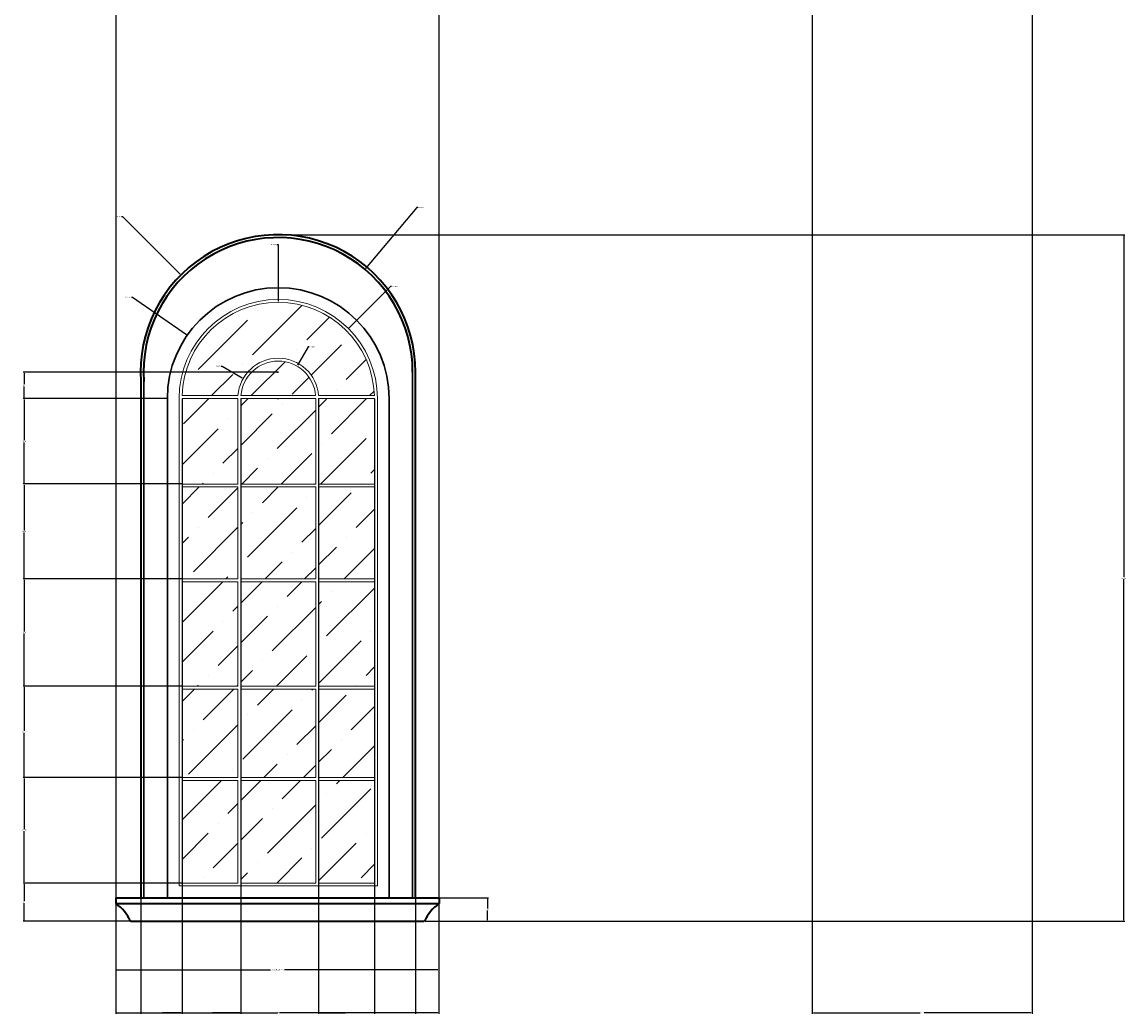
# Model space of a CAD drawing. Units: inches. Extents: x 386 to 708, y 151 to 489.
# Tile 2 of 4: x 520 to 708, y 151 to 320. Entities that reach past the tile are written whole.
import ezdxf

# ---------------------------------------------------------------- set-up
doc = ezdxf.new("R2010")
doc.units = ezdxf.units.IN
doc.header["$MEASUREMENT"] = 0
for name, color, linetype, lineweight in [('A-ANNO-DIMS', 2, 'Continuous', 18), ('A-GLAZ-FRAM', 4, 'Continuous', 30), ('A-GLAZ-PATT', 252, 'Continuous', 13), ('A-GLAZ-SASH', 4, 'Continuous', 18), ('A-GLAZ-SILL', 7, 'Continuous', 35), ('A-GLAZ-TRIM', 7, 'Continuous', 35)]:
    doc.layers.add(name, color=color, linetype=linetype, lineweight=lineweight)
doc.styles.get("Standard").update_dxf_attribs({"font": 'arial.ttf'})
doc.dimstyles.get("Standard").update_dxf_attribs({"dimtxt": 0.18, "dimasz": 0.18, "dimexe": 0.18, "dimexo": 0.0625, "dimgap": 0.09, "dimtad": 0, "dimtih": 1, "dimtoh": 1, "dimdec": 4, "dimzin": 0, "dimdsep": 46, "dimtxsty": 'Standard', "dimcen": 0.09, "dimadec": 0, "dimazin": 0, "dimtfac": 1, "dimtdec": 4, "dimtofl": 0, "dimtmove": 0, "dimatfit": 3, "dimfxl": 1, "dimtolj": 1, "dimtzin": 0, "dimarcsym": 0})

# ---------------------------------------------------------------- blocks, each defined once
blk = doc.blocks.new('WIN-SILL-DOUBLE')
for p, q in [((0, 4), (54.98, 4)), ((0, 4), (0, 3)), ((54.98, 4), (54.98, 3)), ((0, 3), (54.98, 3)), ((2.49, 0), (52.48, 0))]:
    blk.add_line(p, q)
blk.add_lwpolyline([(4.75, 0), (50.49, 0)])
for centre, start, end in [((-4.74, -3.48), 25.6893, 53.8074), ((59.72, -3.48), 126.1926, 154.3107)]:
    blk.add_arc(centre, 8.03, start, end)
blk = doc.blocks.new('*D18')
at = {"layer": 'A-ANNO-DIMS', "color": 0, "lineweight": -2, "transparency": 16777216}
for p, q in [((535.99, 167.19), (535.99, 158.82)), ((590.97, 167.19), (590.97, 158.82)), ((536.17, 159), (562.29, 159)), ((590.79, 159), (564.67, 159))]:
    blk.add_line(p, q, dxfattribs=at)
at = {"layer": 'A-ANNO-DIMS', "color": 0, "transparency": 16777216}
for points in [[(536.17, 159.03), (536.17, 158.97), (535.99, 159)], [(590.79, 159.03), (590.79, 158.97), (590.97, 159)]]:
    blk.add_solid(points, dxfattribs=at)
at = {"layer": 'Defpoints', "color": 0, "transparency": 16777216}
for p in [(535.99, 167.25), (590.97, 167.25), (590.97, 159)]:
    blk.add_point(p, dxfattribs=at)
at = {"layer": 'A-ANNO-DIMS', "color": 0, "transparency": 16777216, "insert": (563.48, 159), "char_height": 0.18, "attachment_point": 5}
blk.add_mtext('\\A1;WIDE SILL 55 TYP.', dxfattribs=at)
blk = doc.blocks.new('*D19')
at = {"layer": 'A-ANNO-DIMS', "color": 0, "lineweight": -2, "transparency": 16777216}
for p, q in [((591.03, 171.25), (599.4, 171.25)), ((599.22, 171.07), (599.22, 169.43)), ((591.03, 167.25), (599.4, 167.25)), ((599.22, 167.43), (599.22, 169.07))]:
    blk.add_line(p, q, dxfattribs=at)
at = {"layer": 'A-ANNO-DIMS', "color": 0, "transparency": 16777216}
for points in [[(599.19, 171.07), (599.25, 171.07), (599.22, 171.25)], [(599.19, 167.43), (599.25, 167.43), (599.22, 167.25)]]:
    blk.add_solid(points, dxfattribs=at)
at = {"layer": 'Defpoints', "color": 0, "transparency": 16777216}
for p in [(590.97, 171.25), (599.22, 171.25), (590.97, 167.25)]:
    blk.add_point(p, dxfattribs=at)
at = {"layer": 'A-ANNO-DIMS', "color": 0, "transparency": 16777216, "insert": (599.22, 169.25), "char_height": 0.18, "attachment_point": 5}
blk.add_mtext('\\A1;4 TYP.', dxfattribs=at)
blk = doc.blocks.new('*D47')
at = {"layer": 'A-ANNO-DIMS', "color": 0, "lineweight": -2, "transparency": 16777216}
for p, q in [((535.99, 370.64), (535.99, 151.47)), ((590.97, 370.64), (590.97, 151.47)), ((536.17, 151.65), (563.09, 151.65)), ((590.79, 151.65), (563.87, 151.65))]:
    blk.add_line(p, q, dxfattribs=at)
at = {"layer": 'A-ANNO-DIMS', "color": 0, "transparency": 16777216}
for points in [[(536.17, 151.68), (536.17, 151.62), (535.99, 151.65)], [(590.79, 151.68), (590.79, 151.62), (590.97, 151.65)]]:
    blk.add_solid(points, dxfattribs=at)
at = {"layer": 'Defpoints', "color": 0, "transparency": 16777216}
for p in [(535.99, 370.7), (590.97, 370.7), (590.97, 151.65)]:
    blk.add_point(p, dxfattribs=at)
at = {"layer": 'A-ANNO-DIMS', "color": 0, "transparency": 16777216, "insert": (563.48, 151.65), "char_height": 0.18, "attachment_point": 5}
blk.add_mtext('\\A1;54.98', dxfattribs=at)
blk = doc.blocks.new('*D51')
at = {"layer": 'A-ANNO-DIMS', "color": 0, "lineweight": -2, "transparency": 16777216}
for p, q in [((654.5, 370.64), (654.5, 151.47)), ((691.9, 370.64), (691.9, 151.47)), ((654.68, 151.65), (672.88, 151.65)), ((691.72, 151.65), (673.53, 151.65))]:
    blk.add_line(p, q, dxfattribs=at)
at = {"layer": 'A-ANNO-DIMS', "color": 0, "transparency": 16777216}
for points in [[(654.68, 151.68), (654.68, 151.62), (654.5, 151.65)], [(691.72, 151.68), (691.72, 151.62), (691.9, 151.65)]]:
    blk.add_solid(points, dxfattribs=at)
at = {"layer": 'Defpoints', "color": 0, "transparency": 16777216}
for p in [(654.5, 370.7), (691.9, 370.7), (691.9, 151.65)]:
    blk.add_point(p, dxfattribs=at)
at = {"layer": 'A-ANNO-DIMS', "color": 0, "transparency": 16777216, "insert": (673.2, 151.65), "char_height": 0.18, "attachment_point": 5}
blk.add_mtext('\\A1;37.4', dxfattribs=at)
blk = doc.blocks.new('*D65')
at = {"layer": 'A-ANNO-DIMS', "color": 0, "lineweight": -2, "transparency": 16777216}
for p, q in [((562.84, 284.1), (707.68, 284.1)), ((707.5, 283.92), (707.5, 225.85)), ((707.5, 167.43), (707.5, 225.49)), ((588.54, 167.25), (707.68, 167.25))]:
    blk.add_line(p, q, dxfattribs=at)
at = {"layer": 'A-ANNO-DIMS', "color": 0, "transparency": 16777216}
for points in [[(707.47, 283.92), (707.53, 283.92), (707.5, 284.1)], [(707.47, 167.43), (707.53, 167.43), (707.5, 167.25)]]:
    blk.add_solid(points, dxfattribs=at)
at = {"layer": 'Defpoints', "color": 0, "transparency": 16777216}
for p in [(562.78, 284.1), (707.5, 284.1), (588.47, 167.25)]:
    blk.add_point(p, dxfattribs=at)
at = {"layer": 'A-ANNO-DIMS', "color": 0, "transparency": 16777216, "insert": (707.5, 225.67), "char_height": 0.18, "attachment_point": 5}
blk.add_mtext('\\A1;116.84', dxfattribs=at)
blk = doc.blocks.new('*D66')
at = {"layer": 'A-ANNO-DIMS', "color": 0, "lineweight": -2, "transparency": 16777216}
for p, q in [((547.17, 173.75), (520.21, 173.75)), ((520.39, 173.57), (520.39, 170.68)), ((520.39, 167.43), (520.39, 170.32)), ((538.42, 167.25), (520.21, 167.25))]:
    blk.add_line(p, q, dxfattribs=at)
at = {"layer": 'A-ANNO-DIMS', "color": 0, "transparency": 16777216}
for points in [[(520.36, 173.57), (520.42, 173.57), (520.39, 173.75)], [(520.36, 167.43), (520.42, 167.43), (520.39, 167.25)]]:
    blk.add_solid(points, dxfattribs=at)
at = {"layer": 'Defpoints', "color": 0, "transparency": 16777216}
for p in [(520.39, 173.75), (547.24, 173.75), (538.49, 167.25)]:
    blk.add_point(p, dxfattribs=at)
at = {"layer": 'A-ANNO-DIMS', "color": 0, "transparency": 16777216, "insert": (520.39, 170.5), "char_height": 0.18, "attachment_point": 5}
blk.add_mtext('\\A1;6.5', dxfattribs=at)
blk = doc.blocks.new('*D67')
at = {"layer": 'A-ANNO-DIMS', "color": 0, "lineweight": -2, "transparency": 16777216}
for p, q in [((547.17, 191.71), (520.21, 191.71)), ((520.39, 191.53), (520.39, 182.91)), ((520.39, 173.93), (520.39, 182.55)), ((547.17, 173.75), (520.21, 173.75))]:
    blk.add_line(p, q, dxfattribs=at)
at = {"layer": 'A-ANNO-DIMS', "color": 0, "transparency": 16777216}
for points in [[(520.36, 191.53), (520.42, 191.53), (520.39, 191.71)], [(520.36, 173.93), (520.42, 173.93), (520.39, 173.75)]]:
    blk.add_solid(points, dxfattribs=at)
at = {"layer": 'Defpoints', "color": 0, "transparency": 16777216}
for p in [(520.39, 191.71), (547.24, 191.71), (547.24, 173.75)]:
    blk.add_point(p, dxfattribs=at)
at = {"layer": 'A-ANNO-DIMS', "color": 0, "transparency": 16777216, "insert": (520.39, 182.73), "char_height": 0.18, "attachment_point": 5}
blk.add_mtext('\\A1;17.955', dxfattribs=at)
blk = doc.blocks.new('*D68')
at = {"layer": 'A-ANNO-DIMS', "color": 0, "lineweight": -2, "transparency": 16777216}
for p, q in [((547.17, 207.26), (520.21, 207.26)), ((520.39, 207.08), (520.39, 199.67)), ((520.39, 191.89), (520.39, 199.3)), ((547.17, 191.71), (520.21, 191.71))]:
    blk.add_line(p, q, dxfattribs=at)
at = {"layer": 'A-ANNO-DIMS', "color": 0, "transparency": 16777216}
for points in [[(520.36, 207.08), (520.42, 207.08), (520.39, 207.26)], [(520.36, 191.89), (520.42, 191.89), (520.39, 191.71)]]:
    blk.add_solid(points, dxfattribs=at)
at = {"layer": 'Defpoints', "color": 0, "transparency": 16777216}
for p in [(520.39, 207.26), (547.24, 207.26), (547.24, 191.71)]:
    blk.add_point(p, dxfattribs=at)
at = {"layer": 'A-ANNO-DIMS', "color": 0, "transparency": 16777216, "insert": (520.39, 199.48), "char_height": 0.18, "attachment_point": 5}
blk.add_mtext('\\A1;15.557', dxfattribs=at)
blk = doc.blocks.new('*D69')
at = {"layer": 'A-ANNO-DIMS', "color": 0, "lineweight": -2, "transparency": 16777216}
for p, q in [((547.17, 225.51), (520.21, 225.51)), ((520.39, 225.33), (520.39, 216.57)), ((520.39, 207.44), (520.39, 216.21)), ((547.17, 207.26), (520.21, 207.26))]:
    blk.add_line(p, q, dxfattribs=at)
at = {"layer": 'A-ANNO-DIMS', "color": 0, "transparency": 16777216}
for points in [[(520.36, 225.33), (520.42, 225.33), (520.39, 225.51)], [(520.36, 207.44), (520.42, 207.44), (520.39, 207.26)]]:
    blk.add_solid(points, dxfattribs=at)
at = {"layer": 'Defpoints', "color": 0, "transparency": 16777216}
for p in [(520.39, 225.51), (547.24, 225.51), (547.24, 207.26)]:
    blk.add_point(p, dxfattribs=at)
at = {"layer": 'A-ANNO-DIMS', "color": 0, "transparency": 16777216, "insert": (520.39, 216.39), "char_height": 0.18, "attachment_point": 5}
blk.add_mtext('\\A1;18.25', dxfattribs=at)
blk = doc.blocks.new('*D70')
at = {"layer": 'A-ANNO-DIMS', "color": 0, "lineweight": -2, "transparency": 16777216}
for p, q in [((547.17, 241.67), (520.21, 241.67)), ((520.39, 241.49), (520.39, 233.77)), ((520.39, 225.69), (520.39, 233.41)), ((547.17, 225.51), (520.21, 225.51))]:
    blk.add_line(p, q, dxfattribs=at)
at = {"layer": 'A-ANNO-DIMS', "color": 0, "transparency": 16777216}
for points in [[(520.36, 241.49), (520.42, 241.49), (520.39, 241.67)], [(520.36, 225.69), (520.42, 225.69), (520.39, 225.51)]]:
    blk.add_solid(points, dxfattribs=at)
at = {"layer": 'Defpoints', "color": 0, "transparency": 16777216}
for p in [(520.39, 241.67), (547.24, 241.67), (547.24, 225.51)]:
    blk.add_point(p, dxfattribs=at)
at = {"layer": 'A-ANNO-DIMS', "color": 0, "transparency": 16777216, "insert": (520.39, 233.59), "char_height": 0.18, "attachment_point": 5}
blk.add_mtext('\\A1;16.155', dxfattribs=at)
blk = doc.blocks.new('*D71')
at = {"layer": 'A-ANNO-DIMS', "color": 0, "lineweight": -2, "transparency": 16777216}
for p, q in [((544.67, 256.21), (520.21, 256.21)), ((520.39, 256.03), (520.39, 249.12)), ((520.39, 241.85), (520.39, 248.76)), ((547.17, 241.67), (520.21, 241.67))]:
    blk.add_line(p, q, dxfattribs=at)
at = {"layer": 'A-ANNO-DIMS', "color": 0, "transparency": 16777216}
for points in [[(520.36, 256.03), (520.42, 256.03), (520.39, 256.21)], [(520.36, 241.85), (520.42, 241.85), (520.39, 241.67)]]:
    blk.add_solid(points, dxfattribs=at)
at = {"layer": 'Defpoints', "color": 0, "transparency": 16777216}
for p in [(520.39, 256.21), (544.74, 256.21), (547.24, 241.67)]:
    blk.add_point(p, dxfattribs=at)
at = {"layer": 'A-ANNO-DIMS', "color": 0, "transparency": 16777216, "insert": (520.39, 248.94), "char_height": 0.18, "attachment_point": 5}
blk.add_mtext('\\A1;14.54', dxfattribs=at)
blk = doc.blocks.new('*D72')
at = {"layer": 'A-ANNO-DIMS', "color": 0, "lineweight": -2, "transparency": 16777216}
for p, q in [((563.52, 260.71), (520.21, 260.71)), ((520.39, 260.53), (520.39, 258.64)), ((520.39, 256.39), (520.39, 258.28)), ((544.67, 256.21), (520.21, 256.21))]:
    blk.add_line(p, q, dxfattribs=at)
at = {"layer": 'A-ANNO-DIMS', "color": 0, "transparency": 16777216}
for points in [[(520.36, 260.53), (520.42, 260.53), (520.39, 260.71)], [(520.36, 256.39), (520.42, 256.39), (520.39, 256.21)]]:
    blk.add_solid(points, dxfattribs=at)
at = {"layer": 'Defpoints', "color": 0, "transparency": 16777216}
for p in [(520.39, 260.71), (563.58, 260.71), (544.74, 256.21)]:
    blk.add_point(p, dxfattribs=at)
at = {"layer": 'A-ANNO-DIMS', "color": 0, "transparency": 16777216, "insert": (520.39, 258.46), "char_height": 0.18, "attachment_point": 5}
blk.add_mtext('\\A1;4.5', dxfattribs=at)
blk = doc.blocks.new('*D73')
at = {"layer": 'A-ANNO-DIMS', "color": 0, "lineweight": -2, "transparency": 16777216}
for p, q in [((540.24, 171.19), (540.24, 151.47)), ((586.99, 171.19), (586.99, 151.47)), ((540.42, 151.65), (563.21, 151.65)), ((586.81, 151.65), (564.01, 151.65))]:
    blk.add_line(p, q, dxfattribs=at)
at = {"layer": 'A-ANNO-DIMS', "color": 0, "transparency": 16777216}
for points in [[(540.42, 151.68), (540.42, 151.62), (540.24, 151.65)], [(586.81, 151.68), (586.81, 151.62), (586.99, 151.65)]]:
    blk.add_solid(points, dxfattribs=at)
at = {"layer": 'Defpoints', "color": 0, "transparency": 16777216}
for p in [(540.24, 171.25), (586.99, 171.25), (586.99, 151.65)]:
    blk.add_point(p, dxfattribs=at)
at = {"layer": 'A-ANNO-DIMS', "color": 0, "transparency": 16777216, "insert": (563.61, 151.65), "char_height": 0.18, "attachment_point": 5}
blk.add_mtext('\\A1;46.75', dxfattribs=at)
blk = doc.blocks.new('*D74')
at = {"layer": 'A-ANNO-DIMS', "color": 0, "lineweight": -2, "transparency": 16777216}
for p, q in [((540.24, 259.03), (540.24, 151.47)), ((547.24, 256.14), (547.24, 151.47)), ((540.42, 151.65), (543.59, 151.65)), ((547.06, 151.65), (543.89, 151.65))]:
    blk.add_line(p, q, dxfattribs=at)
at = {"layer": 'A-ANNO-DIMS', "color": 0, "transparency": 16777216}
for points in [[(540.42, 151.68), (540.42, 151.62), (540.24, 151.65)], [(547.06, 151.68), (547.06, 151.62), (547.24, 151.65)]]:
    blk.add_solid(points, dxfattribs=at)
at = {"layer": 'Defpoints', "color": 0, "transparency": 16777216}
for p in [(540.24, 259.09), (547.24, 256.21), (547.24, 151.65)]:
    blk.add_point(p, dxfattribs=at)
at = {"layer": 'A-ANNO-DIMS', "color": 0, "transparency": 16777216, "insert": (543.74, 151.65), "char_height": 0.18, "attachment_point": 5}
blk.add_mtext('\\A1;7', dxfattribs=at)
blk = doc.blocks.new('*D75')
at = {"layer": 'A-ANNO-DIMS', "color": 0, "lineweight": -2, "transparency": 16777216}
for p, q in [((547.24, 256.14), (547.24, 151.47)), ((557.24, 256.14), (557.24, 151.47)), ((547.42, 151.65), (552.03, 151.65)), ((557.06, 151.65), (552.45, 151.65))]:
    blk.add_line(p, q, dxfattribs=at)
at = {"layer": 'A-ANNO-DIMS', "color": 0, "transparency": 16777216}
for points in [[(547.42, 151.68), (547.42, 151.62), (547.24, 151.65)], [(557.06, 151.68), (557.06, 151.62), (557.24, 151.65)]]:
    blk.add_solid(points, dxfattribs=at)
at = {"layer": 'Defpoints', "color": 0, "transparency": 16777216}
for p in [(547.24, 256.21), (557.24, 256.21), (557.24, 151.65)]:
    blk.add_point(p, dxfattribs=at)
at = {"layer": 'A-ANNO-DIMS', "color": 0, "transparency": 16777216, "insert": (552.24, 151.65), "char_height": 0.18, "attachment_point": 5}
blk.add_mtext('\\A1;10', dxfattribs=at)
blk = doc.blocks.new('*D76')
at = {"layer": 'A-ANNO-DIMS', "color": 0, "lineweight": -2, "transparency": 16777216}
for p, q in [((557.24, 256.14), (557.24, 151.47)), ((570.49, 256.14), (570.49, 151.47)), ((557.42, 151.65), (563.48, 151.65)), ((570.31, 151.65), (564.25, 151.65))]:
    blk.add_line(p, q, dxfattribs=at)
at = {"layer": 'A-ANNO-DIMS', "color": 0, "transparency": 16777216}
for points in [[(557.42, 151.68), (557.42, 151.62), (557.24, 151.65)], [(570.31, 151.68), (570.31, 151.62), (570.49, 151.65)]]:
    blk.add_solid(points, dxfattribs=at)
at = {"layer": 'Defpoints', "color": 0, "transparency": 16777216}
for p in [(557.24, 256.21), (570.49, 256.21), (570.49, 151.65)]:
    blk.add_point(p, dxfattribs=at)
at = {"layer": 'A-ANNO-DIMS', "color": 0, "transparency": 16777216, "insert": (563.86, 151.65), "char_height": 0.18, "attachment_point": 5}
blk.add_mtext('\\A1;13.25', dxfattribs=at)
blk = doc.blocks.new('*D77')
at = {"layer": 'A-ANNO-DIMS', "color": 0, "lineweight": -2, "transparency": 16777216}
for p, q in [((570.49, 256.14), (570.49, 151.47)), ((579.99, 256.14), (579.99, 151.47)), ((570.67, 151.65), (574.98, 151.65)), ((579.81, 151.65), (575.49, 151.65))]:
    blk.add_line(p, q, dxfattribs=at)
at = {"layer": 'A-ANNO-DIMS', "color": 0, "transparency": 16777216}
for points in [[(570.67, 151.68), (570.67, 151.62), (570.49, 151.65)], [(579.81, 151.68), (579.81, 151.62), (579.99, 151.65)]]:
    blk.add_solid(points, dxfattribs=at)
at = {"layer": 'Defpoints', "color": 0, "transparency": 16777216}
for p in [(570.49, 256.21), (579.99, 256.21), (579.99, 151.65)]:
    blk.add_point(p, dxfattribs=at)
at = {"layer": 'A-ANNO-DIMS', "color": 0, "transparency": 16777216, "insert": (575.24, 151.65), "char_height": 0.18, "attachment_point": 5}
blk.add_mtext('\\A1;9.5', dxfattribs=at)
blk = doc.blocks.new('*D88')
at = {"layer": 'A-ANNO-DIMS', "color": 0, "lineweight": -2, "transparency": 16777216}
for p, q in [((536.95, 287.21), (537.13, 287.21)), ((537.13, 287.21), (546.92, 277.4)), ((563.49, 260.71), (563.67, 260.71)), ((563.58, 260.62), (563.58, 260.8))]:
    blk.add_line(p, q, dxfattribs=at)
at = {"layer": 'A-ANNO-DIMS', "color": 0, "transparency": 16777216}
blk.add_solid([(546.94, 277.42), (546.9, 277.37), (547.05, 277.27)], dxfattribs=at)
at = {"layer": 'Defpoints', "color": 0, "transparency": 16777216}
for p in [(547.05, 277.27), (563.58, 260.71)]:
    blk.add_point(p, dxfattribs=at)
at = {"layer": 'A-ANNO-DIMS', "color": 0, "transparency": 16777216, "insert": (536.4, 287.21), "char_height": 0.18, "attachment_point": 5}
blk.add_mtext('\\A1;R23.402', dxfattribs=at)
blk = doc.blocks.new('*D89')
at = {"layer": 'A-ANNO-DIMS', "color": 0, "lineweight": -2, "transparency": 16777216}
for p, q in [((587.17, 288.75), (578.44, 278.37)), ((587.35, 288.75), (587.17, 288.75)), ((563.49, 260.71), (563.67, 260.71)), ((563.58, 260.62), (563.58, 260.8))]:
    blk.add_line(p, q, dxfattribs=at)
at = {"layer": 'A-ANNO-DIMS', "color": 0, "transparency": 16777216}
blk.add_solid([(578.42, 278.39), (578.46, 278.35), (578.32, 278.23)], dxfattribs=at)
at = {"layer": 'Defpoints', "color": 0, "transparency": 16777216}
for p in [(578.32, 278.23), (563.58, 260.71)]:
    blk.add_point(p, dxfattribs=at)
at = {"layer": 'A-ANNO-DIMS', "color": 0, "transparency": 16777216, "insert": (587.9, 288.75), "char_height": 0.18, "attachment_point": 5}
blk.add_mtext('\\A1;R22.902', dxfattribs=at)
blk = doc.blocks.new('*D90')
at = {"layer": 'A-ANNO-DIMS', "color": 0, "lineweight": -2, "transparency": 16777216}
for p, q in [((538.64, 273.46), (538.82, 273.46)), ((538.82, 273.46), (547.97, 267.09)), ((563.52, 256.21), (563.7, 256.21)), ((563.61, 256.12), (563.61, 256.3))]:
    blk.add_line(p, q, dxfattribs=at)
at = {"layer": 'A-ANNO-DIMS', "color": 0, "transparency": 16777216}
blk.add_solid([(547.99, 267.11), (547.95, 267.07), (548.12, 266.99)], dxfattribs=at)
at = {"layer": 'Defpoints', "color": 0, "transparency": 16777216}
for p in [(548.12, 266.99), (563.61, 256.21)]:
    blk.add_point(p, dxfattribs=at)
at = {"layer": 'A-ANNO-DIMS', "color": 0, "transparency": 16777216, "insert": (538.09, 273.46), "char_height": 0.18, "attachment_point": 5}
blk.add_mtext('\\A1;R18.875', dxfattribs=at)
blk = doc.blocks.new('*D91')
at = {"layer": 'A-ANNO-DIMS', "color": 0, "lineweight": -2, "transparency": 16777216}
for p, q in [((582.7, 275.3), (575.67, 268.27)), ((582.88, 275.3), (582.7, 275.3)), ((563.52, 256.21), (563.7, 256.21)), ((563.61, 256.12), (563.61, 256.3))]:
    blk.add_line(p, q, dxfattribs=at)
at = {"layer": 'A-ANNO-DIMS', "color": 0, "transparency": 16777216}
blk.add_solid([(575.65, 268.29), (575.69, 268.24), (575.54, 268.14)], dxfattribs=at)
at = {"layer": 'Defpoints', "color": 0, "transparency": 16777216}
for p in [(575.54, 268.14), (563.61, 256.21)]:
    blk.add_point(p, dxfattribs=at)
at = {"layer": 'A-ANNO-DIMS', "color": 0, "transparency": 16777216, "insert": (583.43, 275.3), "char_height": 0.18, "attachment_point": 5}
blk.add_mtext('\\A1;R16.875', dxfattribs=at)
blk = doc.blocks.new('*D92')
at = {"layer": 'A-ANNO-DIMS', "color": 0, "lineweight": -2, "transparency": 16777216}
for p, q in [((563.43, 282.41), (563.61, 282.41)), ((563.61, 282.41), (563.61, 272.76)), ((563.52, 256.21), (563.7, 256.21)), ((563.61, 256.12), (563.61, 256.3))]:
    blk.add_line(p, q, dxfattribs=at)
at = {"layer": 'A-ANNO-DIMS', "color": 0, "transparency": 16777216}
blk.add_solid([(563.64, 272.76), (563.58, 272.76), (563.61, 272.58)], dxfattribs=at)
at = {"layer": 'Defpoints', "color": 0, "transparency": 16777216}
for p in [(563.61, 272.58), (563.61, 256.21)]:
    blk.add_point(p, dxfattribs=at)
at = {"layer": 'A-ANNO-DIMS', "color": 0, "transparency": 16777216, "insert": (562.88, 282.41), "char_height": 0.18, "attachment_point": 5}
blk.add_mtext('\\A1;R16.375', dxfattribs=at)
blk = doc.blocks.new('*D93')
at = {"layer": 'A-ANNO-DIMS', "color": 0, "lineweight": -2, "transparency": 16777216}
for p, q in [((553.9, 261.7), (554.08, 261.7)), ((554.08, 261.7), (557.5, 259.73)), ((563.52, 256.21), (563.7, 256.21)), ((563.61, 256.12), (563.61, 256.3))]:
    blk.add_line(p, q, dxfattribs=at)
at = {"layer": 'A-ANNO-DIMS', "color": 0, "transparency": 16777216}
blk.add_solid([(557.52, 259.76), (557.49, 259.71), (557.66, 259.64)], dxfattribs=at)
at = {"layer": 'Defpoints', "color": 0, "transparency": 16777216}
for p in [(557.66, 259.64), (563.61, 256.21)]:
    blk.add_point(p, dxfattribs=at)
at = {"layer": 'A-ANNO-DIMS', "color": 0, "transparency": 16777216, "insert": (553.42, 261.7), "char_height": 0.18, "attachment_point": 5}
blk.add_mtext('\\A1;R6.875', dxfattribs=at)
blk = doc.blocks.new('*D94')
at = {"layer": 'A-ANNO-DIMS', "color": 0, "lineweight": -2, "transparency": 16777216}
for p, q in [((568.71, 265.04), (566.89, 261.88)), ((568.89, 265.04), (568.71, 265.04)), ((563.52, 256.21), (563.7, 256.21)), ((563.61, 256.12), (563.61, 256.3))]:
    blk.add_line(p, q, dxfattribs=at)
at = {"layer": 'A-ANNO-DIMS', "color": 0, "transparency": 16777216}
blk.add_solid([(566.86, 261.9), (566.91, 261.87), (566.8, 261.73)], dxfattribs=at)
at = {"layer": 'Defpoints', "color": 0, "transparency": 16777216}
for p in [(566.8, 261.73), (563.61, 256.21)]:
    blk.add_point(p, dxfattribs=at)
at = {"layer": 'A-ANNO-DIMS', "color": 0, "transparency": 16777216, "insert": (569.37, 265.04), "char_height": 0.18, "attachment_point": 5}
blk.add_mtext('\\A1;R6.375', dxfattribs=at)

msp = doc.modelspace()

# ---------------------------------------------------------------- hatches: boundary and pattern name
at = {"layer": 'A-GLAZ-PATT'}
h = msp.add_hatch(dxfattribs=at)
h.set_pattern_fill('ANSI36', color=256, scale=38)
h.paths.add_polyline_path([(569.9858, 191.2056), (557.2368, 191.2056), (557.2368, 173.751), (569.9858, 173.751)])
h.paths.add_polyline_path([(556.7368, 191.2056), (547.2368, 191.2056), (547.2368, 173.751), (556.7368, 173.751)])
h.paths.add_polyline_path([(556.7368, 206.7626), (547.2368, 206.7626), (547.2368, 191.7056), (556.7368, 191.7056)])
h.paths.add_polyline_path([(569.9858, 206.7626), (557.2368, 206.7626), (557.2368, 191.7056), (569.9858, 191.7056)])
h.paths.add_polyline_path([(579.9858, 206.7626), (570.4858, 206.7626), (570.4858, 191.7056), (579.9858, 191.7056)])
h.paths.add_polyline_path([(579.9858, 191.2056), (570.4858, 191.2056), (570.4858, 173.751), (579.9858, 173.751)])
h.paths.add_polyline_path([(579.9858, 225.0121), (570.4858, 225.0121), (570.4858, 207.2626), (579.9858, 207.2626)])
h.paths.add_polyline_path([(569.9858, 225.0121), (557.2368, 225.0121), (557.2368, 207.2626), (569.9858, 207.2626)])
h.paths.add_polyline_path([(556.7368, 225.0121), (547.2368, 225.0121), (547.2368, 207.2626), (556.7368, 207.2626)])
h.paths.add_polyline_path([(556.7368, 241.1674), (547.2368, 241.1674), (547.2368, 225.5121), (556.7368, 225.5121)])
h.paths.add_polyline_path([(569.9858, 241.1674), (557.2368, 241.1674), (557.2368, 225.5121), (569.9858, 225.5121)])
h.paths.add_polyline_path([(579.9858, 241.1674), (570.4858, 241.1674), (570.4858, 225.5121), (579.9858, 225.5121)])
h.paths.add_polyline_path([(579.9858, 256.2066), (570.4858, 256.2066), (570.4858, 241.6674), (579.9858, 241.6674)])
h.paths.add_polyline_path([(569.9858, 256.2066), (557.2368, 256.2066), (557.2368, 241.6674), (569.9858, 241.6674)])
h.paths.add_polyline_path([(556.7368, 256.2066), (547.2368, 256.2066), (547.2368, 241.6674), (556.7368, 241.6674)])
h.paths.add_polyline_path([(570.4676, 256.7066), (579.9782, 256.7066, 0.96991703), (547.2444, 256.7066), (556.755, 256.7066, -0.92973)])
h.paths.add_polyline_path([(557.2564, 256.7066), (569.9662, 256.7066, 0.92441074)], flags=17)
h.paths.add_polyline_path([(578.4858, 393.239), (572.7969, 393.239), (572.7969, 374.702), (578.4858, 374.702)])
h.paths.add_polyline_path([(571.7969, 393.239), (566.1079, 393.239), (566.1079, 374.702), (571.7969, 374.702)])
h.paths.add_polyline_path([(561.1147, 393.239), (555.4258, 393.239), (555.4258, 374.702), (561.1147, 374.702)])
h.paths.add_polyline_path([(554.4258, 393.239), (548.7368, 393.239), (548.7368, 374.702), (554.4258, 374.702)])
h.paths.add_polyline_path([(554.4258, 412.6799), (548.7368, 412.6799), (548.7368, 394.239), (554.4258, 394.239)])
h.paths.add_polyline_path([(561.1147, 412.6799), (555.4258, 412.6799), (555.4258, 394.239), (561.1147, 394.239)])
h.paths.add_polyline_path([(571.7969, 412.6799), (566.1079, 412.6799), (566.1079, 394.239), (571.7969, 394.239)])
h.paths.add_polyline_path([(578.4858, 412.6799), (572.7969, 412.6799), (572.7969, 394.239), (578.4858, 394.239)])
h.paths.add_polyline_path([(578.4858, 432.3276), (572.7969, 432.3276), (572.7969, 413.6799), (578.4858, 413.6799)])
h.paths.add_polyline_path([(571.7969, 432.3276), (566.1079, 432.3276), (566.1079, 413.6799), (571.7969, 413.6799)])
h.paths.add_polyline_path([(561.1147, 432.3276), (555.4258, 432.3276), (555.4258, 413.6799), (561.1147, 413.6799)])
h.paths.add_polyline_path([(554.4258, 432.3276), (548.7368, 432.3276), (548.7368, 413.6799), (554.4258, 413.6799)])
h.paths.add_polyline_path([(554.4258, 451.6577), (548.7368, 451.6577), (548.7368, 433.3276), (554.4258, 433.3276)])
h.paths.add_polyline_path([(561.1147, 451.6577), (555.4258, 451.6577), (555.4258, 433.3276), (561.1147, 433.3276)])
h.paths.add_polyline_path([(571.7969, 451.6577), (566.1079, 451.6577), (566.1079, 433.3276), (571.7969, 433.3276)])
h.paths.add_polyline_path([(578.4858, 451.6577), (572.7969, 451.6577), (572.7969, 433.3276), (578.4858, 433.3276)])
h.paths.add_polyline_path([(672.9386, 451.6577), (667.2497, 451.6577), (667.2497, 433.3276), (672.9386, 433.3276)])
h.paths.add_polyline_path([(679.6276, 451.6577), (673.9386, 451.6577), (673.9386, 433.3276), (679.6276, 433.3276)])
h.paths.add_polyline_path([(679.6276, 432.3276), (673.9386, 432.3276), (673.9386, 413.6799), (679.6276, 413.6799)])
h.paths.add_polyline_path([(672.9386, 432.3276), (667.2497, 432.3276), (667.2497, 413.6799), (672.9386, 413.6799)])
h.paths.add_polyline_path([(672.9386, 412.6799), (667.2497, 412.6799), (667.2497, 394.239), (672.9386, 394.239)])
h.paths.add_polyline_path([(679.6276, 412.6799), (673.9386, 412.6799), (673.9386, 394.239), (679.6276, 394.239)])
h.paths.add_polyline_path([(679.6276, 393.239), (673.9386, 393.239), (673.9386, 374.702), (679.6276, 374.702)])
h.paths.add_polyline_path([(672.9386, 393.239), (667.2497, 393.239), (667.2497, 374.702), (672.9386, 374.702)])

# ---------------------------------------------------------------- linework, layer by layer
at = {"layer": 'A-GLAZ-FRAM'}
for points in [[(540.7368, 260.2066), (540.7368, 171.251)], [(586.4858, 171.251), (586.4858, 260.7066)], [(544.7368, 194.788), (544.7368, 171.251), (582.4858, 171.251), (582.4858, 256.2066)], [(544.7368, 256.2066), (544.7368, 194.788)]]:
    msp.add_lwpolyline(points, dxfattribs=at)
msp.add_arc((563.6113, 256.2066), 18.8745, 0, 180, dxfattribs=at)
at = {"layer": 'A-GLAZ-SASH'}
for points in [[(546.7368, 173.251), (580.4858, 173.251), (580.4858, 256.2066, 1), (546.7368, 256.2066), (546.7368, 194.788)], [(579.9782, 256.7066, 0.96991703), (547.2444, 256.7066)], [(570.4676, 256.7066, 0.92973), (556.755, 256.7066)], [(569.9662, 256.7066, 0.92441074), (557.2564, 256.7066)]]:
    msp.add_lwpolyline(points, format="xyb", dxfattribs=at)
for points in [[(547.2368, 256.2066), (547.2368, 241.6674)], [(556.7368, 256.2066), (547.2368, 256.2066)], [(556.7368, 256.2066), (547.2368, 256.2066)], [(556.755, 256.7066), (547.2444, 256.7066)], [(556.7368, 256.2066), (556.7368, 241.6674)], [(563.1147, 256.2066), (557.2368, 256.2066)], [(557.2368, 256.2066), (557.2368, 241.6674)], [(569.9858, 256.2066), (557.2368, 256.2066)], [(569.9662, 256.7066), (557.2564, 256.7066)], [(569.9858, 256.2066), (564.1079, 256.2066)], [(569.9858, 241.6674), (569.9858, 256.2066)], [(579.9782, 256.7066), (570.4676, 256.7066)], [(579.9858, 256.2066), (570.4858, 256.2066)], [(579.9858, 256.2066), (570.4858, 256.2066)], [(570.4858, 241.6674), (570.4858, 256.2066)], [(579.9858, 241.6674), (579.9858, 256.2066)], [(556.7368, 241.6674), (547.2368, 241.6674)], [(556.7368, 241.1674), (547.2368, 241.1674)], [(547.2368, 241.1674), (547.2368, 225.5121)], [(556.7368, 241.1674), (556.7368, 225.5121)], [(569.9858, 241.6674), (557.2368, 241.6674)], [(569.9858, 241.1674), (557.2368, 241.1674)], [(557.2368, 241.1674), (557.2368, 225.5121)], [(569.9858, 241.1674), (564.1155, 241.1674)], [(569.9858, 225.5121), (569.9858, 241.1674)], [(579.9858, 241.6674), (570.4858, 241.6674)], [(579.9858, 241.1674), (570.4858, 241.1674)], [(579.9858, 241.1674), (570.4858, 241.1674)], [(570.4858, 225.5121), (570.4858, 241.1674)], [(579.9858, 225.5121), (579.9858, 241.1674)], [(556.7368, 225.5121), (547.2368, 225.5121)], [(569.9858, 225.5121), (557.2368, 225.5121)], [(579.9858, 225.5121), (570.4858, 225.5121)], [(547.2368, 225.0121), (547.2368, 207.2626)], [(556.7368, 225.0121), (547.2368, 225.0121)], [(556.7368, 225.0121), (556.7368, 207.2626)], [(557.2368, 225.0121), (557.2368, 207.2626)], [(569.9858, 225.0121), (557.2368, 225.0121)], [(569.9858, 225.0121), (564.1155, 225.0121)], [(569.9858, 207.2626), (569.9858, 225.0121)], [(579.9935, 225.0121), (570.4858, 225.0121)], [(579.9935, 225.0121), (570.4858, 225.0121)], [(570.4858, 207.2626), (570.4858, 225.0121)], [(579.9858, 207.2626), (579.9858, 225.0121)], [(556.7368, 207.2626), (547.2368, 207.2626)], [(556.7368, 206.7626), (547.2368, 206.7626)], [(547.2368, 206.7626), (547.2368, 191.7056)], [(556.7368, 206.7626), (556.7368, 191.7056)], [(569.9858, 207.2626), (557.2368, 207.2626)], [(569.9858, 206.7626), (557.2368, 206.7626)], [(557.2368, 206.7626), (557.2368, 191.7056)], [(569.9858, 206.7626), (564.6155, 206.7626)], [(569.9858, 191.7056), (569.9858, 206.7626)], [(579.9858, 207.2626), (570.4858, 207.2626)], [(579.9858, 206.7626), (570.4858, 206.7626)], [(579.9858, 206.7626), (570.4858, 206.7626)], [(570.4858, 191.7056), (570.4858, 206.7626)], [(579.9858, 191.7056), (579.9858, 206.7626)], [(580.4935, 206.7626), (580.4858, 206.7626)], [(580.4935, 206.7626), (580.4858, 206.7626)], [(546.7368, 194.788), (546.7368, 173.251), (563.1147, 173.251)], [(556.7368, 191.7056), (547.2368, 191.7056)], [(569.9858, 191.7056), (557.2368, 191.7056)], [(579.9858, 191.7056), (570.4858, 191.7056)], [(547.2368, 191.2056), (547.2368, 173.751), (556.7368, 173.751)], [(556.7368, 191.2056), (547.2368, 191.2056)], [(556.7368, 191.2056), (556.7368, 173.751)], [(557.2368, 191.2056), (557.2368, 173.751)], [(569.9858, 191.2056), (557.2368, 191.2056)], [(569.9858, 191.2056), (564.6155, 191.2056)], [(569.9858, 173.751), (569.9858, 191.2056)], [(570.4858, 173.751), (570.4858, 191.2056)], [(579.9858, 191.2056), (570.4858, 191.2056)], [(579.9858, 191.2056), (570.4858, 191.2056)], [(570.4858, 173.751), (579.9858, 173.751), (579.9858, 191.2056)], [(580.4935, 191.2056), (580.4858, 191.2056)], [(580.4935, 191.2056), (580.4858, 191.2056)], [(557.2368, 173.751), (569.9858, 173.751)]]:
    msp.add_lwpolyline(points, dxfattribs=at)
at = {"layer": 'A-GLAZ-TRIM'}
for points in [[(586.9858, 171.251), (586.9858, 260.7066)], [(540.2368, 259.0935), (540.2368, 171.251)]]:
    msp.add_lwpolyline(points, dxfattribs=at)
for radius in [23.4023, 22.9023]:
    msp.add_arc((563.5835, 260.7066), radius, 0, 183.952524, dxfattribs=at)

# ---------------------------------------------------------------- block references
at = {"layer": 'A-GLAZ-SILL'}
msp.add_blockref('WIN-SILL-DOUBLE', (535.991, 167.251), dxfattribs=at)

# ---------------------------------------------------------------- dimensions: what is measured, and where the dimension line sits
at = {"layer": 'A-ANNO-DIMS'}
for base, p1, p2, override, picture, middle in [((590.9688, 151.651), (535.9906, 370.702), (590.9688, 370.702), {"dimdec": 2, "dimlfac": 1, "dimrnd": 0, "dimzin": 0, "dimdsep": 46, "dimlunit": 2}, '*D47', (563.4797, 151.651)), ((691.9, 151.651), (654.5034, 370.702), (691.9, 370.702), {"dimdec": 1, "dimlfac": 1, "dimrnd": 0, "dimzin": 0, "dimdsep": 46, "dimlunit": 2}, '*D51', (673.2017, 151.651)), ((547.2368, 151.651), (540.2368, 259.0935), (547.2368, 256.2066), {"dimdec": 0, "dimlfac": 1, "dimrnd": 0, "dimzin": 0, "dimdsep": 46, "dimlunit": 2}, '*D74', (543.7368, 151.651)), ((557.2368, 151.651), (547.2368, 256.2066), (557.2368, 256.2066), {"dimdec": 0, "dimlfac": 1, "dimrnd": 0, "dimzin": 0, "dimdsep": 46, "dimlunit": 2}, '*D75', (552.2368, 151.651)), ((570.4858, 151.651), (557.2368, 256.2066), (570.4858, 256.2066), {"dimdec": 2, "dimlfac": 1, "dimrnd": 0, "dimzin": 0, "dimdsep": 46, "dimlunit": 2}, '*D76', (563.8613, 151.651)), ((579.9858, 151.651), (570.4858, 256.2066), (579.9858, 256.2066), {"dimdec": 1, "dimlfac": 1, "dimrnd": 0, "dimzin": 0, "dimdsep": 46, "dimlunit": 2}, '*D77', (575.2358, 151.651)), ((586.9858, 151.651), (540.2368, 171.251), (586.9858, 171.251), {"dimdec": 2, "dimlfac": 1, "dimrnd": 0, "dimzin": 0, "dimdsep": 46, "dimlunit": 2}, '*D73', (563.6113, 151.651))]:
    dim = msp.add_linear_dim(base=base, p1=p1, p2=p2, dimstyle='Standard', override=override, dxfattribs=at)
    dim.commit()
    dim.dimension.update_dxf_attribs({"geometry": picture, "text_midpoint": middle})
for center, mpoint, picture, middle in [((563.5835, 260.7066), (578.3239, 278.2349), '*D89', (587.897, 288.7518)), ((563.5835, 260.7066), (547.0495, 277.2686), '*D88', (536.4002, 287.2057)), ((563.6113, 256.2066), (563.611, 272.5812), '*D92', (562.8804, 282.4059)), ((563.6113, 256.2066), (575.5436, 268.1386), '*D91', (583.4333, 275.2977)), ((563.6113, 256.2066), (548.1183, 266.987), '*D90', (538.0921, 273.4552)), ((563.6113, 256.2066), (566.7982, 261.7273), '*D94', (569.3708, 265.0398)), ((563.6113, 256.2066), (557.6572, 259.6429), '*D93', (553.4242, 261.7046))]:
    dim = msp.add_radius_dim(center=center, mpoint=mpoint, dimstyle='Standard', override={"dimdec": 3, "dimlfac": 1, "dimrnd": 0, "dimzin": 0, "dimdsep": 46, "dimlunit": 2}, dxfattribs=at)
    dim.commit()
    dim.dimension.update_dxf_attribs({"geometry": picture, "text_midpoint": middle, "dimtype": 164})
for base, p1, p2, override, picture, middle in [((707.5, 284.0951), (588.4739, 167.251), (562.7764, 284.0951), {"dimdec": 2, "dimlfac": 1, "dimrnd": 0, "dimzin": 0, "dimdsep": 46, "dimlunit": 2}, '*D65', (707.5, 225.673)), ((520.3906, 260.7066), (544.7368, 256.2066), (563.5835, 260.7066), {"dimdec": 1, "dimlfac": 1, "dimrnd": 0, "dimzin": 0, "dimdsep": 46, "dimlunit": 2}, '*D72', (520.3906, 258.4566)), ((520.3906, 256.2066), (547.2368, 241.6674), (544.7368, 256.2066), {"dimdec": 2, "dimlfac": 1, "dimrnd": 0, "dimzin": 0, "dimdsep": 46, "dimlunit": 2}, '*D71', (520.3906, 248.937)), ((520.3906, 241.6674), (547.2368, 225.5121), (547.2368, 241.6674), {"dimdec": 3, "dimlfac": 1, "dimrnd": 0, "dimzin": 0, "dimdsep": 46, "dimlunit": 2}, '*D70', (520.3906, 233.5898)), ((520.3906, 225.5121), (547.2368, 207.2626), (547.2368, 225.5121), {"dimdec": 2, "dimlfac": 1, "dimrnd": 0, "dimzin": 0, "dimdsep": 46, "dimlunit": 2}, '*D69', (520.3906, 216.3874)), ((520.3906, 207.2626), (547.2368, 191.7056), (547.2368, 207.2626), {"dimdec": 3, "dimlfac": 1, "dimrnd": 0, "dimzin": 0, "dimdsep": 46, "dimlunit": 2}, '*D68', (520.3906, 199.4841)), ((520.3906, 191.7056), (547.2368, 173.751), (547.2368, 191.7056), {"dimdec": 3, "dimlfac": 1, "dimrnd": 0, "dimzin": 0, "dimdsep": 46, "dimlunit": 2}, '*D67', (520.3906, 182.7283)), ((520.3906, 173.751), (538.4855, 167.251), (547.2368, 173.751), {"dimdec": 1, "dimlfac": 1, "dimrnd": 0, "dimzin": 0, "dimdsep": 46, "dimlunit": 2}, '*D66', (520.3906, 170.501))]:
    dim = msp.add_linear_dim(base=base, p1=p1, p2=p2, angle=90, dimstyle='Standard', override=override, dxfattribs=at)
    dim.commit()
    dim.dimension.update_dxf_attribs({"geometry": picture, "text_midpoint": middle})
dim = msp.add_linear_dim(base=(599.2156, 171.251), p1=(590.9688, 167.251), p2=(590.9688, 171.251), angle=90, text='<> TYP.', dimstyle='Standard', override={"dimdec": 0, "dimlfac": 1, "dimrnd": 0, "dimzin": 0, "dimdsep": 46, "dimlunit": 2}, dxfattribs=at)
dim.commit()
dim.dimension.update_dxf_attribs({"geometry": '*D19', "text_midpoint": (599.2156, 169.251)})
dim = msp.add_linear_dim(base=(590.9688, 159.0043), p1=(535.9906, 167.251), p2=(590.9688, 167.251), text='WIDE SILL <> TYP.', dimstyle='Standard', override={"dimdec": 0, "dimlfac": 1, "dimrnd": 0, "dimzin": 0, "dimdsep": 46, "dimlunit": 2}, dxfattribs=at)
dim.commit()
dim.dimension.update_dxf_attribs({"geometry": '*D18', "text_midpoint": (563.4797, 159.0043)})

doc.saveas('drawing.dxf')
